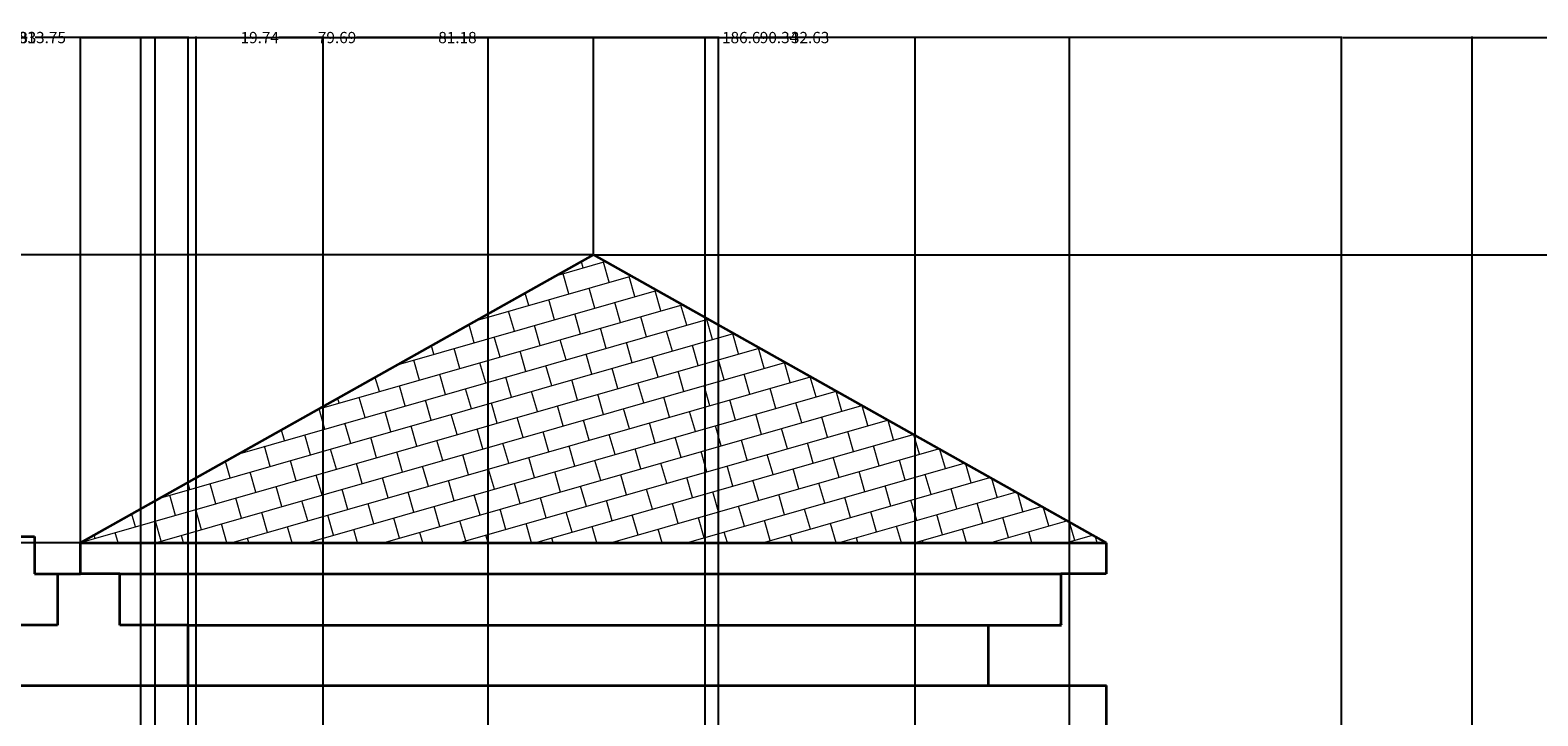
# Model space of a CAD drawing. Units: inches. Extents: x -17 to 741, y 7 to 490.
# Tile 6 of 8: x 254 to 489, y 383 to 490. Entities that reach past the tile are written whole.
import ezdxf

# ---------------------------------------------------------------- set-up
doc = ezdxf.new("R2010")
doc.units = ezdxf.units.IN
doc.header["$MEASUREMENT"] = 0
for name, color, linetype, lineweight in [('A-ANNO-DIMS', 2, 'Continuous', 18), ('A-ROOF', 7, 'Continuous', 35), ('A-ROOF-PATT', 8, 'Continuous', 13)]:
    doc.layers.add(name, color=color, linetype=linetype, lineweight=lineweight)
doc.styles.get("Standard").update_dxf_attribs({"font": 'arial.ttf'})
doc.dimstyles.get("Standard").update_dxf_attribs({"dimtxt": 1.75, "dimasz": 0.18, "dimexe": 0.18, "dimexo": 0.0625, "dimgap": 0.09, "dimtad": 0, "dimtih": 1, "dimtoh": 1, "dimdec": 4, "dimzin": 0, "dimdsep": 46, "dimlunit": 4, "dimtxsty": 'Standard', "dimcen": 0.09, "dimadec": 0, "dimazin": 0, "dimtfac": 1, "dimtdec": 4, "dimtofl": 0, "dimtmove": 0, "dimatfit": 3, "dimfxl": 1, "dimtolj": 1, "dimtzin": 0, "dimarcsym": 0})

# ---------------------------------------------------------------- blocks, each defined once
blk = doc.blocks.new('*D37')
at = {"layer": 'A-ANNO-DIMS', "color": 0, "lineweight": -2, "transparency": 16777216}
for p, q in [((20.52, 396.95), (20.52, 14.58)), ((553.43, 51.95), (553.43, 14.58)), ((20.7, 14.76), (283.93, 14.76)), ((553.25, 14.76), (290.02, 14.76))]:
    blk.add_line(p, q, dxfattribs=at)
at = {"layer": 'A-ANNO-DIMS', "color": 0, "transparency": 16777216}
for points in [[(20.7, 14.79), (20.7, 14.73), (20.52, 14.76)], [(553.25, 14.79), (553.25, 14.73), (553.43, 14.76)]]:
    blk.add_solid(points, dxfattribs=at)
at = {"layer": 'Defpoints', "color": 0, "transparency": 16777216}
for p in [(20.52, 397.01), (553.43, 52.01), (553.43, 14.76)]:
    blk.add_point(p, dxfattribs=at)
at = {"layer": 'A-ANNO-DIMS', "color": 0, "transparency": 16777216, "insert": (286.97, 14.76), "char_height": 1.75, "attachment_point": 5}
blk.add_mtext('\\A1;532.9', dxfattribs=at)
blk = doc.blocks.new('*D38')
at = {"layer": 'A-ANNO-DIMS', "color": 0, "lineweight": -2, "transparency": 16777216}
for p, q in [((341.83, 454.57), (723.06, 454.57)), ((722.88, 454.39), (722.88, 254.27)), ((722.88, 52.19), (722.88, 252.31)), ((553.49, 52.01), (723.06, 52.01))]:
    blk.add_line(p, q, dxfattribs=at)
at = {"layer": 'A-ANNO-DIMS', "color": 0, "transparency": 16777216}
for points in [[(722.85, 454.39), (722.91, 454.39), (722.88, 454.57)], [(722.85, 52.19), (722.91, 52.19), (722.88, 52.01)]]:
    blk.add_solid(points, dxfattribs=at)
at = {"layer": 'Defpoints', "color": 0, "transparency": 16777216}
for p in [(341.77, 454.57), (722.88, 454.57), (553.43, 52.01)]:
    blk.add_point(p, dxfattribs=at)
at = {"layer": 'A-ANNO-DIMS', "color": 0, "transparency": 16777216, "insert": (722.88, 253.29), "char_height": 1.75, "attachment_point": 5}
blk.add_mtext('\\A1;402.6', dxfattribs=at)
blk = doc.blocks.new('*D43')
at = {"layer": 'A-ANNO-DIMS', "color": 0, "lineweight": -2, "transparency": 16777216}
for p, q in [((241, 410.88), (241, 488.55)), ((241.18, 488.37), (247.8, 488.37)), ((261.9, 488.37), (255.28, 488.37)), ((262.08, 409.88), (262.08, 488.55))]:
    blk.add_line(p, q, dxfattribs=at)
at = {"layer": 'A-ANNO-DIMS', "color": 0, "transparency": 16777216}
for points in [[(241.18, 488.4), (241.18, 488.34), (241, 488.37)], [(261.9, 488.4), (261.9, 488.34), (262.08, 488.37)]]:
    blk.add_solid(points, dxfattribs=at)
at = {"layer": 'Defpoints', "color": 0, "transparency": 16777216}
for p in [(262.08, 488.37), (241, 410.82), (262.08, 409.82)]:
    blk.add_point(p, dxfattribs=at)
at = {"layer": 'A-ANNO-DIMS', "color": 0, "transparency": 16777216, "insert": (251.54, 488.37), "char_height": 1.75, "attachment_point": 5}
blk.add_mtext('\\A1;21.083', dxfattribs=at)
blk = doc.blocks.new('*D44')
at = {"layer": 'A-ANNO-DIMS', "color": 0, "lineweight": -2, "transparency": 16777216}
for p, q in [((262.08, 409.88), (262.08, 488.55)), ((262.26, 488.37), (298.89, 488.37)), ((341.59, 488.37), (304.96, 488.37)), ((341.77, 454.63), (341.77, 488.55))]:
    blk.add_line(p, q, dxfattribs=at)
at = {"layer": 'A-ANNO-DIMS', "color": 0, "transparency": 16777216}
for points in [[(262.26, 488.4), (262.26, 488.34), (262.08, 488.37)], [(341.59, 488.4), (341.59, 488.34), (341.77, 488.37)]]:
    blk.add_solid(points, dxfattribs=at)
at = {"layer": 'Defpoints', "color": 0, "transparency": 16777216}
for p in [(341.77, 488.37), (341.77, 454.57), (262.08, 409.82)]:
    blk.add_point(p, dxfattribs=at)
at = {"layer": 'A-ANNO-DIMS', "color": 0, "transparency": 16777216, "insert": (301.93, 488.37), "char_height": 1.75, "attachment_point": 5}
blk.add_mtext('\\A1;79.69', dxfattribs=at)
blk = doc.blocks.new('*D45')
at = {"layer": 'A-ANNO-DIMS', "color": 0, "lineweight": -2, "transparency": 16777216}
for p, q in [((341.71, 454.57), (-13.46, 454.57)), ((-13.28, 454.39), (-13.28, 433.18)), ((-13.28, 410), (-13.28, 431.22)), ((262.02, 409.82), (-13.46, 409.82))]:
    blk.add_line(p, q, dxfattribs=at)
at = {"layer": 'A-ANNO-DIMS', "color": 0, "transparency": 16777216}
for points in [[(-13.31, 454.39), (-13.25, 454.39), (-13.28, 454.57)], [(-13.31, 410), (-13.25, 410), (-13.28, 409.82)]]:
    blk.add_solid(points, dxfattribs=at)
at = {"layer": 'Defpoints', "color": 0, "transparency": 16777216}
for p in [(-13.28, 454.57), (341.77, 454.57), (262.08, 409.82)]:
    blk.add_point(p, dxfattribs=at)
at = {"layer": 'A-ANNO-DIMS', "color": 0, "transparency": 16777216, "insert": (-13.28, 432.2), "char_height": 1.75, "attachment_point": 5}
blk.add_mtext('\\A1;44.75', dxfattribs=at)
blk = doc.blocks.new('*D52')
at = {"layer": 'A-ANNO-DIMS', "color": 0, "lineweight": -2, "transparency": 16777216}
for p, q in [((239.94, 113.25), (239.94, 488.55)), ((240.12, 488.37), (253.76, 488.37)), ((273.51, 488.37), (259.86, 488.37)), ((273.69, 113.25), (273.69, 488.55))]:
    blk.add_line(p, q, dxfattribs=at)
at = {"layer": 'A-ANNO-DIMS', "color": 0, "transparency": 16777216}
for points in [[(240.12, 488.4), (240.12, 488.34), (239.94, 488.37)], [(273.51, 488.4), (273.51, 488.34), (273.69, 488.37)]]:
    blk.add_solid(points, dxfattribs=at)
at = {"layer": 'Defpoints', "color": 0, "transparency": 16777216}
for p in [(273.69, 488.37), (239.94, 113.19), (273.69, 113.19)]:
    blk.add_point(p, dxfattribs=at)
at = {"layer": 'A-ANNO-DIMS', "color": 0, "transparency": 16777216, "insert": (256.81, 488.37), "char_height": 1.75, "attachment_point": 5}
blk.add_mtext('\\A1;33.75', dxfattribs=at)
blk = doc.blocks.new('*D53')
at = {"layer": 'A-ANNO-DIMS', "color": 0, "lineweight": -2, "transparency": 16777216}
for p, q in [((271.44, 167.89), (271.44, 488.55)), ((271.62, 488.37), (361.78, 488.37)), ((457.87, 488.37), (367.7, 488.37)), ((458.05, 167.89), (458.05, 488.55))]:
    blk.add_line(p, q, dxfattribs=at)
at = {"layer": 'A-ANNO-DIMS', "color": 0, "transparency": 16777216}
for points in [[(271.62, 488.4), (271.62, 488.34), (271.44, 488.37)], [(457.87, 488.4), (457.87, 488.34), (458.05, 488.37)]]:
    blk.add_solid(points, dxfattribs=at)
at = {"layer": 'Defpoints', "color": 0, "transparency": 16777216}
for p in [(458.05, 488.37), (271.44, 167.83), (458.05, 167.83)]:
    blk.add_point(p, dxfattribs=at)
at = {"layer": 'A-ANNO-DIMS', "color": 0, "transparency": 16777216, "insert": (364.74, 488.37), "char_height": 1.75, "attachment_point": 5}
blk.add_mtext('\\A1;186.6', dxfattribs=at)
blk = doc.blocks.new('*D54')
at = {"layer": 'A-ANNO-DIMS', "color": 0, "lineweight": -2, "transparency": 16777216}
for p, q in [((458.05, 167.89), (458.05, 488.55)), ((458.23, 488.37), (502.69, 488.37)), ((553.25, 488.37), (508.78, 488.37)), ((553.43, 52.07), (553.43, 488.55))]:
    blk.add_line(p, q, dxfattribs=at)
at = {"layer": 'A-ANNO-DIMS', "color": 0, "transparency": 16777216}
for points in [[(458.23, 488.4), (458.23, 488.34), (458.05, 488.37)], [(553.25, 488.4), (553.25, 488.34), (553.43, 488.37)]]:
    blk.add_solid(points, dxfattribs=at)
at = {"layer": 'Defpoints', "color": 0, "transparency": 16777216}
for p in [(553.43, 488.37), (458.05, 167.83), (553.43, 52.01)]:
    blk.add_point(p, dxfattribs=at)
at = {"layer": 'A-ANNO-DIMS', "color": 0, "transparency": 16777216, "insert": (505.74, 488.37), "char_height": 1.75, "attachment_point": 5}
blk.add_mtext('\\A1;95.38', dxfattribs=at)
blk = doc.blocks.new('*D56')
at = {"layer": 'A-ANNO-DIMS', "color": 0, "lineweight": -2, "transparency": 16777216}
for p, q in [((225.47, 260.11), (225.47, 488.55)), ((225.65, 488.37), (249.25, 488.37)), ((278.6, 488.37), (255, 488.37)), ((278.78, 243.73), (278.78, 488.55))]:
    blk.add_line(p, q, dxfattribs=at)
at = {"layer": 'A-ANNO-DIMS', "color": 0, "transparency": 16777216}
for points in [[(225.65, 488.4), (225.65, 488.34), (225.47, 488.37)], [(278.6, 488.4), (278.6, 488.34), (278.78, 488.37)]]:
    blk.add_solid(points, dxfattribs=at)
at = {"layer": 'Defpoints', "color": 0, "transparency": 16777216}
for p in [(278.78, 488.37), (225.47, 260.05), (278.78, 243.67)]:
    blk.add_point(p, dxfattribs=at)
at = {"layer": 'A-ANNO-DIMS', "color": 0, "transparency": 16777216, "insert": (252.12, 488.37), "char_height": 1.75, "attachment_point": 5}
blk.add_mtext('\\A1;53.31', dxfattribs=at)
blk = doc.blocks.new('*D57')
at = {"layer": 'A-ANNO-DIMS', "color": 0, "lineweight": -2, "transparency": 16777216}
for p, q in [((325.44, 243.73), (325.44, 488.55)), ((325.62, 488.37), (367.57, 488.37)), ((415.6, 488.37), (373.65, 488.37)), ((415.78, 260.11), (415.78, 488.55))]:
    blk.add_line(p, q, dxfattribs=at)
at = {"layer": 'A-ANNO-DIMS', "color": 0, "transparency": 16777216}
for points in [[(325.62, 488.4), (325.62, 488.34), (325.44, 488.37)], [(415.6, 488.4), (415.6, 488.34), (415.78, 488.37)]]:
    blk.add_solid(points, dxfattribs=at)
at = {"layer": 'Defpoints', "color": 0, "transparency": 16777216}
for p in [(415.78, 488.37), (415.78, 260.05), (325.44, 243.67)]:
    blk.add_point(p, dxfattribs=at)
at = {"layer": 'A-ANNO-DIMS', "color": 0, "transparency": 16777216, "insert": (370.61, 488.37), "char_height": 1.75, "attachment_point": 5}
blk.add_mtext('\\A1;90.34', dxfattribs=at)
blk = doc.blocks.new('*D60')
at = {"layer": 'A-ANNO-DIMS', "color": 0, "lineweight": -2, "transparency": 16777216}
for p, q in [((280.05, 68.56), (280.05, 488.55)), ((280.23, 488.37), (286.96, 488.37)), ((299.61, 488.37), (292.87, 488.37)), ((299.79, 76.07), (299.79, 488.55))]:
    blk.add_line(p, q, dxfattribs=at)
at = {"layer": 'A-ANNO-DIMS', "color": 0, "transparency": 16777216}
for points in [[(280.23, 488.4), (280.23, 488.34), (280.05, 488.37)], [(299.61, 488.4), (299.61, 488.34), (299.79, 488.37)]]:
    blk.add_solid(points, dxfattribs=at)
at = {"layer": 'Defpoints', "color": 0, "transparency": 16777216}
for p in [(299.79, 488.37), (299.79, 76.01), (280.05, 68.49)]:
    blk.add_point(p, dxfattribs=at)
at = {"layer": 'A-ANNO-DIMS', "color": 0, "transparency": 16777216, "insert": (289.92, 488.37), "char_height": 1.75, "attachment_point": 5}
blk.add_mtext('\\A1;19.74', dxfattribs=at)
blk = doc.blocks.new('*D65')
at = {"layer": 'A-ANNO-DIMS', "color": 0, "lineweight": -2, "transparency": 16777216}
for p, q in [((478.32, 220.07), (478.32, 488.55)), ((478.5, 488.37), (513.01, 488.37)), ((553.25, 488.37), (518.74, 488.37)), ((553.43, 308.03), (553.43, 488.55))]:
    blk.add_line(p, q, dxfattribs=at)
at = {"layer": 'A-ANNO-DIMS', "color": 0, "transparency": 16777216}
for points in [[(478.5, 488.4), (478.5, 488.34), (478.32, 488.37)], [(553.25, 488.4), (553.25, 488.34), (553.43, 488.37)]]:
    blk.add_solid(points, dxfattribs=at)
at = {"layer": 'Defpoints', "color": 0, "transparency": 16777216}
for p in [(553.43, 488.37), (553.43, 307.97), (478.32, 220.01)]:
    blk.add_point(p, dxfattribs=at)
at = {"layer": 'A-ANNO-DIMS', "color": 0, "transparency": 16777216, "insert": (515.87, 488.37), "char_height": 1.75, "attachment_point": 5}
blk.add_mtext('\\A1;75.11', dxfattribs=at)
blk = doc.blocks.new('*D67')
at = {"layer": 'A-ANNO-DIMS', "color": 0, "lineweight": -2, "transparency": 16777216}
for p, q in [((359.14, 243.73), (359.14, 488.55)), ((359.32, 488.37), (372.41, 488.37)), ((391.59, 488.37), (378.49, 488.37)), ((391.77, 243.73), (391.77, 488.55))]:
    blk.add_line(p, q, dxfattribs=at)
at = {"layer": 'A-ANNO-DIMS', "color": 0, "transparency": 16777216}
for points in [[(359.32, 488.4), (359.32, 488.34), (359.14, 488.37)], [(391.59, 488.4), (391.59, 488.34), (391.77, 488.37)]]:
    blk.add_solid(points, dxfattribs=at)
at = {"layer": 'Defpoints', "color": 0, "transparency": 16777216}
for p in [(391.77, 488.37), (359.14, 243.67), (391.77, 243.67)]:
    blk.add_point(p, dxfattribs=at)
at = {"layer": 'A-ANNO-DIMS', "color": 0, "transparency": 16777216, "insert": (375.45, 488.37), "char_height": 1.75, "attachment_point": 5}
blk.add_mtext('\\A1;32.63', dxfattribs=at)
blk = doc.blocks.new('*D68')
at = {"layer": 'A-ANNO-DIMS', "color": 0, "lineweight": -2, "transparency": 16777216}
for p, q in [((280.05, 61.98), (280.05, 488.55)), ((280.23, 488.37), (317.59, 488.37)), ((361.04, 488.37), (323.68, 488.37)), ((361.22, 61.98), (361.22, 488.55))]:
    blk.add_line(p, q, dxfattribs=at)
at = {"layer": 'A-ANNO-DIMS', "color": 0, "transparency": 16777216}
for points in [[(280.23, 488.4), (280.23, 488.34), (280.05, 488.37)], [(361.04, 488.4), (361.04, 488.34), (361.22, 488.37)]]:
    blk.add_solid(points, dxfattribs=at)
at = {"layer": 'Defpoints', "color": 0, "transparency": 16777216}
for p in [(361.22, 488.37), (280.05, 61.91), (361.22, 61.91)]:
    blk.add_point(p, dxfattribs=at)
at = {"layer": 'A-ANNO-DIMS', "color": 0, "transparency": 16777216, "insert": (320.64, 488.37), "char_height": 1.75, "attachment_point": 5}
blk.add_mtext('\\A1;81.18', dxfattribs=at)

msp = doc.modelspace()

# ---------------------------------------------------------------- hatches: boundary and pattern name
at = {"layer": 'A-ROOF-PATT'}
h = msp.add_hatch(dxfattribs=at)
h.set_pattern_fill('BRICK', color=256, scale=13, angle=16)
h.paths.add_polyline_path([(341.7687, 454.5717), (262.0821, 409.8217), (421.4553, 409.8217)])
h.paths.add_polyline_path([(553.4286, 379.9466), (515.96, 379.9466), (493.0961, 379.9466), (553.4286, 307.9703)])

# ---------------------------------------------------------------- linework, layer by layer
at = {"layer": 'A-ROOF'}
for p, q in [((262.0821, 409.8217), (341.7687, 454.5717)), ((341.7687, 454.5717), (421.4553, 409.8217)), ((20.5169, 410.8173), (254.8926, 410.8173)), ((254.8926, 410.8173), (254.8926, 405.0149)), ((262.0821, 405.0149), (262.0821, 409.8217)), ((262.0821, 409.8217), (421.4553, 409.8217)), ((421.4553, 409.8217), (421.4553, 405.0149)), ((254.8926, 405.0149), (262.0821, 405.0149)), ((258.4874, 405.0149), (258.4874, 397.0087)), ((268.165, 405.0149), (262.0821, 405.0149)), ((268.165, 397.0087), (268.165, 405.0149)), ((268.165, 405.0149), (414.3956, 405.0149)), ((414.3956, 405.0149), (414.3956, 397.3726)), ((421.4553, 405.0149), (414.3956, 405.0149)), ((258.4874, 397.0087), (20.5169, 397.0087)), ((278.7803, 397.0087), (268.165, 397.0087)), ((278.7803, 387.669), (278.7803, 397.0087)), ((278.7803, 397.0087), (403.1051, 397.0087)), ((403.1051, 397.0087), (403.1051, 387.669)), ((403.1051, 397.0087), (414.5302, 397.0087)), ((414.5302, 397.0087), (414.3956, 397.3726)), ((53.4591, 387.669), (421.4932, 387.669)), ((421.4932, 379.9466), (421.4932, 387.669))]:
    msp.add_line(p, q, dxfattribs=at)

# ---------------------------------------------------------------- dimensions: what is measured, and where the dimension line sits
at = {"layer": 'A-ANNO-DIMS'}
for base, p1, p2, override, picture, middle in [((278.7803, 488.3717), (225.4694, 260.0479), (278.7803, 243.669), {"dimdec": 2, "dimlfac": 1, "dimrnd": 0, "dimzin": 0, "dimdsep": 46, "dimlunit": 2}, '*D56', (252.1249, 488.3717)), ((273.6893, 488.3717), (239.9367, 113.1863), (273.6893, 113.1863), {"dimdec": 2, "dimlfac": 1, "dimrnd": 0, "dimzin": 0, "dimdsep": 46, "dimlunit": 2}, '*D52', (256.813, 488.3717)), ((262.0821, 488.3717), (240.9987, 410.8173), (262.0821, 409.8217), {"dimdec": 3, "dimlfac": 1, "dimrnd": 0, "dimzin": 0, "dimdsep": 46, "dimlunit": 2}, '*D43', (251.5404, 488.3717)), ((341.7687, 488.3717), (262.0821, 409.8217), (341.7687, 454.5717), {"dimdec": 2, "dimlfac": 1, "dimrnd": 0, "dimzin": 0, "dimdsep": 46, "dimlunit": 2}, '*D44', (301.9254, 488.3717)), ((458.0494, 488.3717), (271.4367, 167.8255), (458.0494, 167.8255), {"dimdec": 1, "dimlfac": 1, "dimrnd": 0, "dimzin": 0, "dimdsep": 46, "dimlunit": 2}, '*D53', (364.743, 488.3717)), ((299.7867, 488.3717), (280.0481, 68.493), (299.7867, 76.0082), {"dimdec": 2, "dimlfac": 1, "dimrnd": 0, "dimzin": 0, "dimdsep": 46, "dimlunit": 2}, '*D60', (289.9174, 488.3717)), ((361.2234, 488.3717), (280.0481, 61.9147), (361.2234, 61.9147), {"dimdec": 2, "dimlfac": 1, "dimrnd": 0, "dimzin": 0, "dimdsep": 46, "dimlunit": 2}, '*D68', (320.6357, 488.3717)), ((415.7774, 488.3717), (325.441, 243.669), (415.7774, 260.0479), {"dimdec": 2, "dimlfac": 1, "dimrnd": 0, "dimzin": 0, "dimdsep": 46, "dimlunit": 2}, '*D57', (370.6092, 488.3717)), ((391.7691, 488.3717), (359.1364, 243.669), (391.7691, 243.669), {"dimdec": 2, "dimlfac": 1, "dimrnd": 0, "dimzin": 0, "dimdsep": 46, "dimlunit": 2}, '*D67', (375.4527, 488.3717)), ((553.4286, 488.3717), (458.0494, 167.8255), (553.4286, 52.0082), {"dimdec": 2, "dimlfac": 1, "dimrnd": 0, "dimzin": 0, "dimdsep": 46, "dimlunit": 2}, '*D54', (505.739, 488.3717)), ((553.4286, 488.3717), (478.3168, 220.0082), (553.4286, 307.9703), {"dimdec": 2, "dimlfac": 1, "dimrnd": 0, "dimzin": 0, "dimdsep": 46, "dimlunit": 2}, '*D65', (515.8727, 488.3717)), ((553.4286, 14.7597), (20.5169, 397.0087), (553.4286, 52.0082), {"dimdec": 1, "dimlfac": 1, "dimrnd": 0, "dimzin": 0, "dimdsep": 46, "dimlunit": 2}, '*D37', (286.9727, 14.7597))]:
    dim = msp.add_linear_dim(base=base, p1=p1, p2=p2, dimstyle='Standard', override=override, dxfattribs=at)
    dim.commit()
    dim.dimension.update_dxf_attribs({"geometry": picture, "text_midpoint": middle})
for base, p1, override, picture, middle in [((-13.2831, 454.5717), (262.0821, 409.8217), {"dimdec": 2, "dimlfac": 1, "dimrnd": 0, "dimzin": 0, "dimdsep": 46, "dimlunit": 2}, '*D45', (-13.2831, 432.1967)), ((722.8826, 454.5717), (553.4286, 52.0082), {"dimdec": 1, "dimlfac": 1, "dimrnd": 0, "dimzin": 0, "dimdsep": 46, "dimlunit": 2}, '*D38', (722.8826, 253.2899))]:
    dim = msp.add_linear_dim(base=base, p1=p1, p2=(341.7687, 454.5717), angle=90, dimstyle='Standard', override=override, dxfattribs=at)
    dim.commit()
    dim.dimension.update_dxf_attribs({"geometry": picture, "text_midpoint": middle})

doc.saveas('drawing.dxf')
